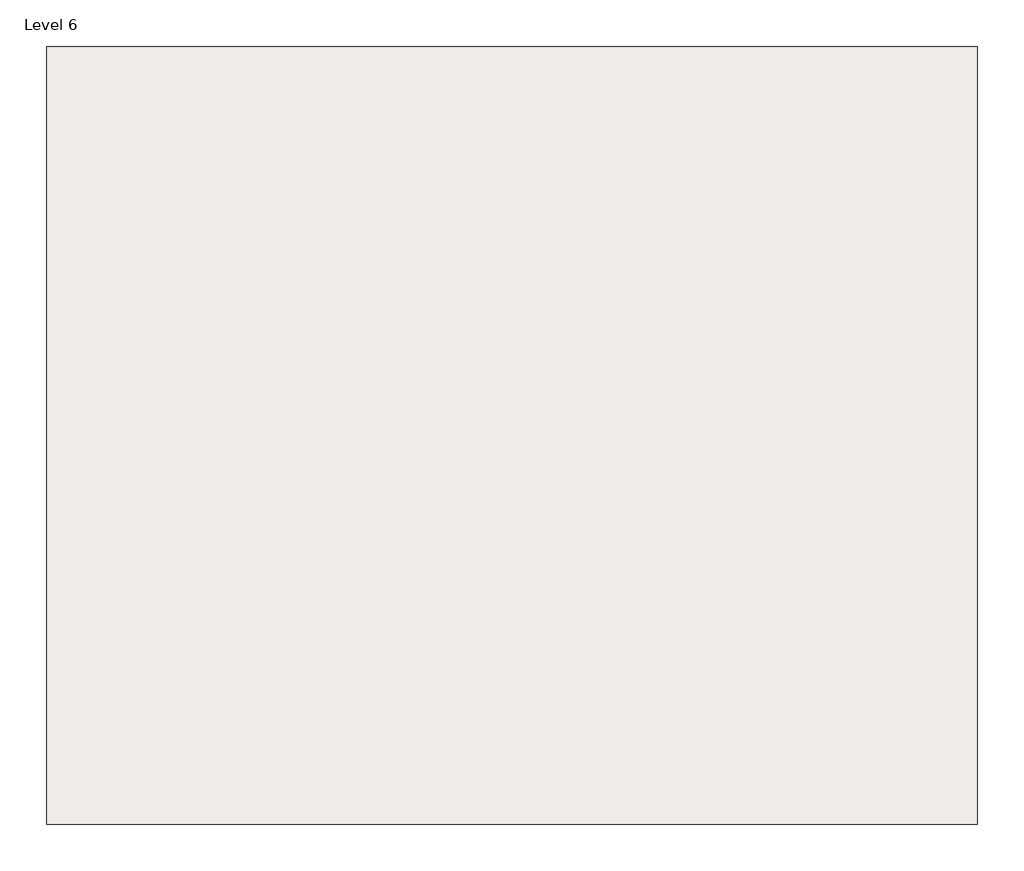
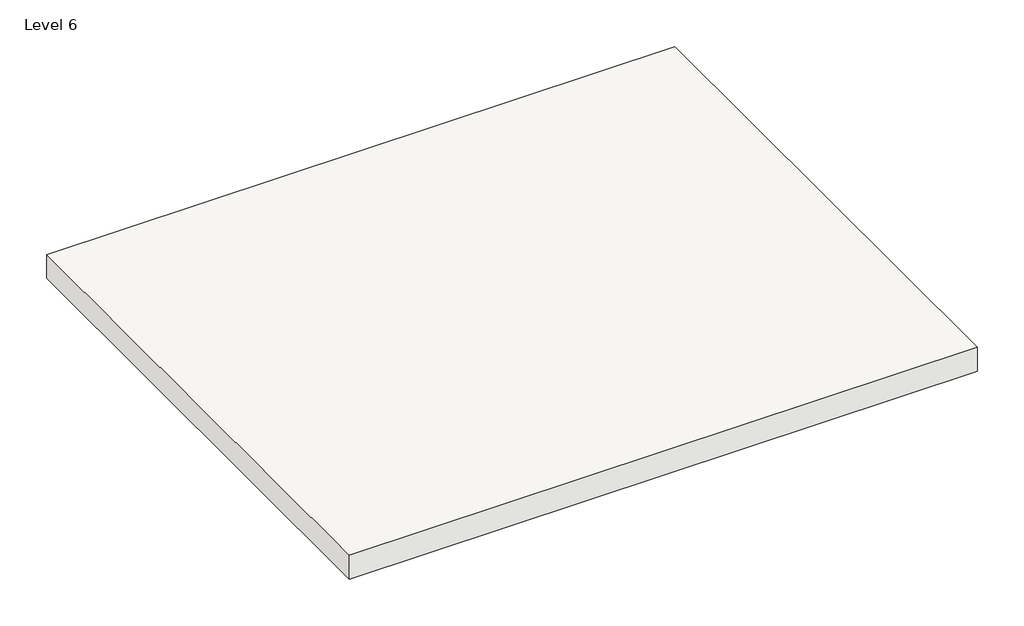
# One storey: 1 roof.
"""IFC4 building model written with IfcOpenShell, lengths in millimetres."""

from ifc_helpers import new_model, si_unit, frame, origin, place, context, project, spatial, polyline, outline, extrude, element, save

model = new_model("IFC4")

# Units and contexts
model_context = context("Model", 3, world=origin())
ifc_project = project(units=[si_unit("LENGTHUNIT", "METRE", prefix="MILLI")], contexts=[model_context])

# Site, building, storey
site = spatial("IfcSite", under=ifc_project)
building = spatial("IfcBuilding", under=site)
storey = spatial("IfcBuildingStorey", under=building, Name="Level 6", Elevation=12801.6)

# Roof
placement = place(None, origin())
element("IfcRoof", 1, ObjectType="Generic - 12\"", at=placement, inside=storey, context=model_context, shape_type="SweptSolid", body=[
    extrude(outline(polyline([(-2067.514408, 4166.8022623), (1735.6084916, 4166.8022623), (1735.6084916, 989.5652728), (-2067.514408, 989.5652728), (-2067.514408, 4166.8022623)])), frame((0.0, 0.0, 12649.2), z_axis=(0.0, 0.0, 1.0), x_axis=(1.0, 0.0, 0.0)), (0.0, 0.0, 1.0), 152.4),
])

save(model, "model.ifc")

# Revit data of these elements
# Type "Generic - 12\""
#   Assembly Code = "B1020"
#   Layers, outside or top first: 0' - 6" no material (function 1)
# Element 1 (IfcRoof, "Generic - 12\"")
#   built-in parameter 1001705 = 42 (stored number, unit not read)
#   built-in parameter 1001701 = -0.5 (stored number, unit not read)
#   built-in parameter 1001710 = 33615
#   Phase Created = New Construction
#   Materials on its faces: "Blanket", "Default Roof"
# Materials
#   "Blanket": class "System", colour RGB 59 0 1, transparency 0, Cost = 0
#   "Default Roof": colour RGB 88 101 114, transparency 0, Cost = 0
